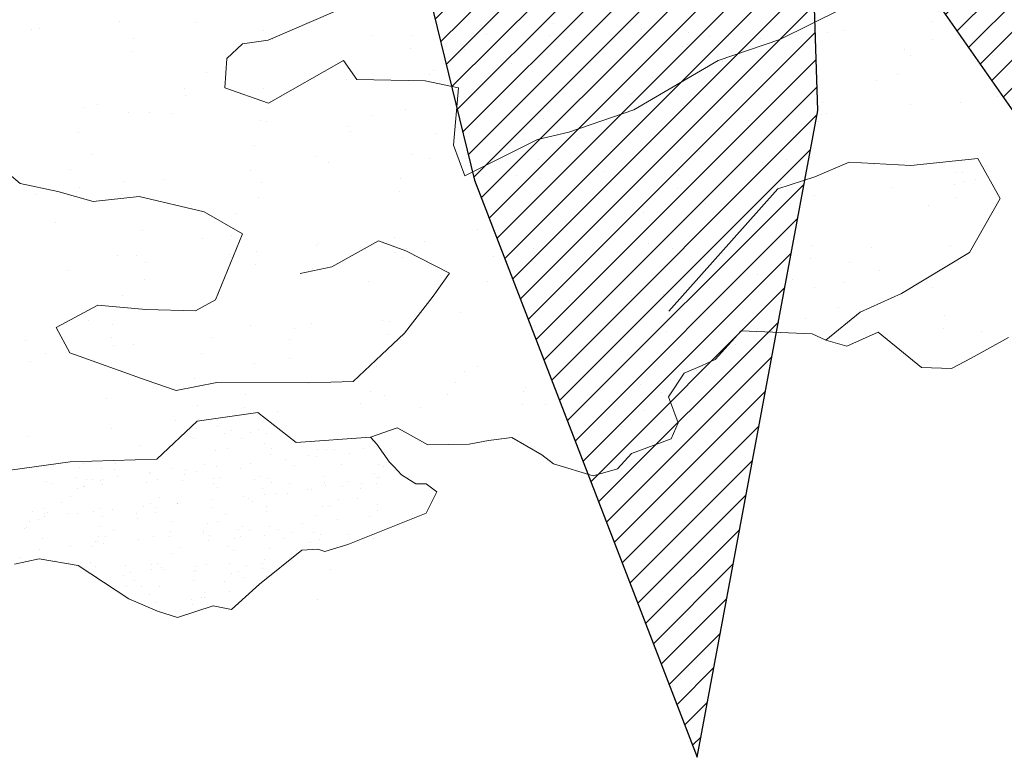
# Model space of a CAD drawing. Units: inches. Extents: x 1986 to 21484, y -1816 to 2016.
# Tile 52 of 85: x 3664.13 to 3671.752, y 1865.089 to 1870.798. Entities that reach past the tile are written whole.
import ezdxf

# ---------------------------------------------------------------- set-up
doc = ezdxf.new("R2010")
doc.units = ezdxf.units.IN
doc.layers.add('L-PLNT', color=84, linetype='Continuous', lineweight=13)
doc.layers.add('vfolhas', color=114, linetype='Continuous', lineweight=5)
for name, color, linetype in [('vfolha', 72, 'Continuous'), ('vfolha2', 110, 'Continuous'), ('vfolhas2', 102, 'Continuous')]:
    doc.layers.add(name, color=color, linetype=linetype)
pattern_1 = [(45, (-2446.5133113, 50.986076), (-0.004419417382, 0.004419417382), [])]

# ---------------------------------------------------------------- blocks, each defined once
blk = doc.blocks.new('arbusto_PB_verde_grande')
at = {"layer": 'vfolha2'}
h = blk.add_hatch(dxfattribs=at)
h.set_pattern_fill('ANSI31', color=256, scale=0.05, style=0)
h.set_pattern_definition(pattern_1)
h.paths.add_polyline_path([(-0.18963, 0.29704), (-0.08553, 0.20192), (-0.10785, 0.25007), (-0.13202, 0.31865), (-0.25096, 0.48479), (-0.44952, 0.5505), (-0.37946, 0.43789)])
h.paths.add_polyline_path([(0.07911, -0.4071), (0.08214, -0.50631), (0.17255, -0.6355), (0.18428, -0.44151), (0.14904, -0.29177), (0.02625, -0.03934), (0.03527, -0.25376)])
at = {"layer": 'vfolhas'}
h = blk.add_hatch(dxfattribs=at)
h.set_pattern_fill('ANSI31', color=256, scale=0.05, style=0)
h.set_pattern_definition(pattern_1)
h.paths.add_polyline_path([(-0.07279, 0.50669), (-0.18085, 0.65063), (-0.2334, 0.67253), (-0.20712, 0.53176), (-0.10785, 0.25007), (0.02625, -0.03934), (0.00028, 0.09048), (0.00816, 0.16241), (-0.04939, 0.29079)])
h.paths.add_polyline_path([(0.09902, 0.41929), (0.09372, 0.26573), (0.07906, 0.18814), (0.15506, 0.36901), (0.26606, 0.5505), (0.28356, 0.63504), (0.2485, 0.68819), (0.25145, 0.63504), (0.20178, 0.54426)])
h.paths.add_polyline_path([(0.12295, 0.24073), (0.047, 0.06233), (0.02625, -0.03934), (0.11122, 0.04358), (0.18428, 0.09364), (0.27478, 0.19376), (0.3215, 0.25323), (0.44129, 0.38467), (0.47634, 0.57866), (0.41789, 0.45347), (0.28939, 0.30954)])
h.paths.add_polyline_path([(0.58145, -0.03779), (0.70707, 0.01536), (0.78591, 0.04667), (0.74796, 0.06549), (0.62818, 0.08423), (0.52595, 0.09048), (0.39745, 0.04358), (0.02625, -0.03934), (0.25728, -0.03154), (0.43834, -0.0347)])
h.paths.add_polyline_path([(0.52022, -0.03647), (0.43834, -0.0347), (0.25728, -0.03154), (0.02625, -0.03934), (0.17964, -0.08515), (0.53768, -0.13167), (0.69541, -0.15357), (0.78591, -0.07852), (0.70413, -0.10042)])
h.paths.add_polyline_path([(0.27189, -0.21929), (0.14922, -0.14107), (0.02625, -0.03934), (0.15794, -0.31007), (0.29522, -0.42585), (0.41789, -0.49157), (0.56396, -0.56669), (0.5114, -0.48532), (0.39456, -0.34139)])
h.paths.add_polyline_path([(-0.05818, -0.47591), (-0.02312, -0.61984), (0.047, -0.80134), (0.08494, -0.59794), (0.07911, -0.4071), (0.03527, -0.25376), (0.02625, -0.03934), (-0.03773, -0.26001)])
h.paths.add_polyline_path([(-0.24218, 0.14054), (-0.11073, 0.06858), (0.02625, -0.03934), (-0.04235, 0.10871), (-0.21007, 0.23757), (-0.36485, 0.33145), (-0.47874, 0.40341), (-0.54303, 0.46288), (-0.49041, 0.33145), (-0.39408, 0.22192)])
at = {"layer": 'vfolha'}
for p, q in [((0.08494, -0.59794), (0.07911, -0.4071)), ((0.047, -0.80134), (0.08494, -0.59794)), ((-0.02312, -0.61984), (0.047, -0.80134))]:
    blk.add_line(p, q, dxfattribs=at)
at = {"layer": 'vfolha2'}
blk.add_line((0.08214, -0.50631), (0.17255, -0.6355), dxfattribs=at)
at = {"layer": 'vfolhas2'}
blk.add_line((-0.05818, -0.47591), (-0.02312, -0.61984), dxfattribs=at)
blk = doc.blocks.new('PLANT-SHRUB')
for p, q in [((2172.6241, 1903.2659), (2172.9437, 1903.1835)), ((2172.9437, 1903.1835), (2173.1087, 1903.1371)), ((2173.1087, 1903.1371), (2173.2736, 1902.9723)), ((2172.7447, 1903.0859), (2172.7447, 1903.0859)), ((2173.2736, 1902.9723), (2173.3303, 1902.5448)), ((2172.9389, 1902.8692), (2172.9389, 1902.8692)), ((2172.8652, 1902.8017), (2172.8652, 1902.8017)), ((2172.7867, 1902.5845), (2172.7867, 1902.5845)), ((2172.3937, 1902.5791), (2171.9348, 1902.4358)), ((2172.3937, 1902.5791), (2172.3937, 1902.5791)), ((2172.9961, 1902.4501), (2172.3937, 1902.5791)), ((2172.5128, 1902.5757), (2172.5128, 1902.5757)), ((2173.3303, 1902.5448), (2173.583, 1902.457)), ((2171.9348, 1902.4358), (2171.8488, 1902.0919)), ((2171.9348, 1902.4358), (2171.9348, 1902.4358)), ((2172.4674, 1902.4372), (2172.4674, 1902.4372)), ((2173.3259, 1902.3355), (2172.9961, 1902.4501)), ((2173.583, 1902.457), (2173.6695, 1902.312)), ((2173.583, 1902.457), (2173.583, 1902.457)), ((2173.6695, 1902.312), (2173.3259, 1902.3355)), ((2173.6695, 1902.312), (2173.7128, 1902.2026)), ((2172.9948, 1902.2058), (2172.9948, 1902.2058)), ((2171.8432, 1902.1697), (2171.8432, 1902.1697)), ((2171.9724, 1902.2009), (2171.9724, 1902.2009)), ((2172.0512, 1902.1424), (2172.0512, 1902.1424)), ((2172.1799, 1902.198), (2172.1799, 1902.198)), ((2173.4246, 1902.1957), (2173.4246, 1902.1957)), ((2173.7128, 1902.2026), (2174.0978, 1901.8122)), ((2171.8488, 1902.0919), (2172.2647, 1901.7766)), ((2171.8488, 1902.0919), (2171.8488, 1902.0919)), ((2172.0114, 1902.0906), (2172.0114, 1902.0906)), ((2172.046, 1902.051), (2172.046, 1902.051)), ((2172.1197, 1902.1185), (2172.1197, 1902.1185)), ((2172.3762, 1902.0996), (2172.3762, 1902.0996)), ((2173.256, 1902.0884), (2173.256, 1902.0884)), ((2173.6688, 1902.0864), (2173.6688, 1902.0864)), ((2172.919, 1902.0281), (2172.919, 1902.0281)), ((2173.1271, 1902.0007), (2173.1271, 1902.0007)), ((2174.8579, 1901.7985), (2174.9403, 1901.9952)), ((2174.9403, 1901.9952), (2175.0639, 1902.0501)), ((2175.0639, 1902.0501), (2175.3661, 1901.922)), ((2173.452, 1901.9579), (2173.452, 1901.9579)), ((2175.3661, 1901.922), (2175.5264, 1901.9357)), ((2175.5264, 1901.9357), (2175.7004, 1901.8442)), ((2171.4082, 1901.8444), (2171.4082, 1901.8444)), ((2173.9948, 1901.8865), (2173.9948, 1901.8865)), ((2174.0978, 1901.8122), (2174.3954, 1901.8351)), ((2174.2029, 1901.8591), (2174.2029, 1901.8591)), ((2174.3954, 1901.8351), (2174.5008, 1901.7985)), ((2175.7004, 1901.8442), (2175.8617, 1901.568)), ((2172.2647, 1901.7766), (2172.5945, 1901.4326)), ((2172.2647, 1901.7766), (2172.2647, 1901.7766)), ((2172.4877, 1901.8056), (2172.4877, 1901.8056)), ((2173.3211, 1901.7678), (2173.3211, 1901.7678)), ((2173.5338, 1901.7922), (2173.5338, 1901.7922)), ((2174.0978, 1901.8122), (2174.0978, 1901.8122)), ((2174.5008, 1901.7985), (2174.6427, 1901.7481)), ((2174.5278, 1901.8163), (2174.5278, 1901.8163)), ((2174.5562, 1901.7971), (2174.5562, 1901.7971)), ((2174.6427, 1901.7481), (2174.8579, 1901.7985)), ((2171.6482, 1901.6865), (2171.6482, 1901.6865)), ((2173.2475, 1901.7003), (2173.2475, 1901.7003)), ((2174.8703, 1901.7356), (2174.8703, 1901.7356)), ((2175.0707, 1901.7448), (2175.0707, 1901.7448)), ((2175.2787, 1901.7175), (2175.2787, 1901.7175)), ((2175.6036, 1901.6747), (2175.6036, 1901.6747)), ((2171.2193, 1901.586), (2171.2193, 1901.586)), ((2172.4639, 1901.5837), (2172.4639, 1901.5837)), ((2173.7085, 1901.5815), (2173.7085, 1901.5815)), ((2174.9532, 1901.5792), (2174.9532, 1901.5792)), ((2175.8617, 1901.568), (2175.88, 1901.4537)), ((2175.88, 1901.4537), (2175.9578, 1901.1974)), ((2171.3005, 1901.3679), (2171.3005, 1901.3679)), ((2171.9472, 1901.4308), (2171.9472, 1901.4308)), ((2172.5945, 1901.4326), (2172.867, 1901.3323)), ((2172.9696, 1901.4357), (2172.9696, 1901.4357)), ((2174.0491, 1901.3968), (2174.0491, 1901.3968)), ((2174.5226, 1901.417), (2174.5226, 1901.417)), ((2175.0953, 1901.3835), (2175.0953, 1901.3835)), ((2171.2268, 1901.3004), (2171.2268, 1901.3004)), ((2172.8497, 1901.3357), (2172.8497, 1901.3357)), ((2172.867, 1901.3323), (2173.1395, 1901.2034)), ((2173.1395, 1901.2034), (2174.4016, 1901.318)), ((2174.4016, 1901.318), (2174.4016, 1901.318)), ((2174.4489, 1901.3495), (2174.4489, 1901.3495)), ((2171.4747, 1901.1835), (2171.4747, 1901.1835)), ((2171.6827, 1901.1561), (2171.6827, 1901.1561)), ((2171.8572, 1901.1972), (2171.8572, 1901.1972)), ((2173.1018, 1901.1949), (2173.1018, 1901.1949)), ((2174.3464, 1901.1927), (2174.3464, 1901.1927)), ((2175.591, 1901.1904), (2175.591, 1901.1904)), ((2175.9578, 1901.1974), (2176.1044, 1901.0922)), ((2176.6676, 1901.1059), (2176.8415, 1901.17)), ((2176.8415, 1901.17), (2177.4505, 1900.9321)), ((2176.8415, 1901.17), (2176.8415, 1901.17)), ((2171.383, 1901.0744), (2171.383, 1901.0744)), ((2171.6886, 1901.0898), (2171.6886, 1901.0898)), ((2172.0077, 1901.1133), (2172.0077, 1901.1133)), ((2172.9332, 1901.0876), (2172.9332, 1901.0876)), ((2174.1779, 1901.0853), (2174.1779, 1901.0853)), ((2175.4225, 1901.083), (2175.4225, 1901.083)), ((2175.7241, 1901.0662), (2175.7241, 1901.0662)), ((2176.1044, 1901.0922), (2176.2326, 1901.0099)), ((2176.6859, 1901.0053), (2176.6676, 1901.1059)), ((2177.9118, 1901.0785), (2177.9118, 1901.0785)), ((2172.4625, 1901.0355), (2172.4625, 1901.0355)), ((2172.502, 1901.0171), (2172.502, 1901.0171)), ((2172.5505, 1901.0418), (2172.5505, 1901.0418)), ((2172.7586, 1901.0144), (2172.7586, 1901.0144)), ((2173.5087, 1901.0221), (2173.5087, 1901.0221)), ((2174.0511, 1900.985), (2174.0511, 1900.985)), ((2174.5311, 1901.027), (2174.5311, 1901.027)), ((2175.6105, 1900.9881), (2175.6105, 1900.9881)), ((2175.6504, 1900.9987), (2175.6504, 1900.9987)), ((2176.2326, 1901.0099), (2176.4707, 1900.7948)), ((2176.7454, 1900.9504), (2176.6859, 1901.0053)), ((2177.2732, 1901.034), (2177.2732, 1901.034)), ((2172.4283, 1900.9496), (2172.4283, 1900.9496)), ((2173.0835, 1900.9717), (2173.0835, 1900.9717)), ((2176.7774, 1900.8223), (2176.7454, 1900.9504)), ((2177.4505, 1900.9321), (2177.6154, 1900.8497)), ((2177.6791, 1900.9797), (2177.6791, 1900.9797)), ((2173.6264, 1900.9002), (2173.6264, 1900.9002)), ((2173.8344, 1900.8728), (2173.8344, 1900.8728)), ((2177.0704, 1900.8682), (2177.0704, 1900.8682)), ((2177.0998, 1900.8952), (2177.0998, 1900.8952)), ((2177.182, 1900.8875), (2177.182, 1900.8875)), ((2177.392, 1900.8776), (2177.392, 1900.8776)), ((2177.6154, 1900.8497), (2177.6428, 1900.7994)), ((2174.1593, 1900.83), (2174.1593, 1900.83)), ((2174.7022, 1900.7585), (2174.7022, 1900.7585)), ((2176.4707, 1900.7948), (2176.5302, 1900.6027)), ((2176.7774, 1900.7399), (2176.7774, 1900.8223)), ((2177.5804, 1900.7549), (2177.5804, 1900.7549)), ((2177.6428, 1900.7994), (2177.739, 1900.7216)), ((2174.9102, 1900.7312), (2174.9102, 1900.7312)), ((2175.2351, 1900.6884), (2175.2351, 1900.6884)), ((2176.7545, 1900.5203), (2176.7774, 1900.6896)), ((2176.7774, 1900.6896), (2176.7774, 1900.7399)), ((2176.8372, 1900.6844), (2176.8372, 1900.6844)), ((2176.9112, 1900.7224), (2176.9112, 1900.7224)), ((2176.9255, 1900.7154), (2176.9255, 1900.7154)), ((2176.9659, 1900.7376), (2176.9659, 1900.7376)), ((2177.0819, 1900.68), (2177.0819, 1900.68)), ((2177.1493, 1900.7229), (2177.1493, 1900.7229)), ((2177.3748, 1900.7395), (2177.3748, 1900.7395)), ((2177.5509, 1900.7279), (2177.5509, 1900.7279)), ((2177.5798, 1900.6791), (2177.5798, 1900.6791)), ((2177.6472, 1900.722), (2177.6472, 1900.722)), ((2177.739, 1900.7216), (2178.1577, 1900.6883)), ((2178.1577, 1900.6883), (2178.4507, 1900.6838)), ((2178.1577, 1900.6883), (2178.1577, 1900.6883)), ((2178.4507, 1900.6838), (2178.5331, 1900.5648)), ((2171.9221, 1900.6607), (2171.9221, 1900.6607)), ((2172.9445, 1900.6656), (2172.9445, 1900.6656)), ((2173.7034, 1900.6663), (2173.7034, 1900.6663)), ((2174.0239, 1900.6267), (2174.0239, 1900.6267)), ((2175.0701, 1900.6134), (2175.0701, 1900.6134)), ((2175.2526, 1900.6342), (2175.2526, 1900.6342)), ((2175.778, 1900.6169), (2175.778, 1900.6169)), ((2176.0925, 1900.6183), (2176.0925, 1900.6183)), ((2176.5302, 1900.6027), (2176.5531, 1900.534)), ((2176.8519, 1900.6479), (2176.8519, 1900.6479)), ((2176.9204, 1900.6735), (2176.9204, 1900.6735)), ((2177.0504, 1900.6564), (2177.0504, 1900.6564)), ((2177.2675, 1900.6278), (2177.2675, 1900.6278)), ((2177.3507, 1900.6168), (2177.3507, 1900.6168)), ((2178.061, 1900.6146), (2178.061, 1900.6146)), ((2178.0776, 1900.6782), (2178.0776, 1900.6782)), ((2172.0305, 1900.5851), (2172.0305, 1900.5851)), ((2172.1411, 1900.5829), (2172.1411, 1900.5829)), ((2173.3857, 1900.5806), (2173.3857, 1900.5806)), ((2173.6298, 1900.5988), (2173.6298, 1900.5988)), ((2174.6304, 1900.5784), (2174.6304, 1900.5784)), ((2175.875, 1900.5761), (2175.875, 1900.5761)), ((2175.986, 1900.5895), (2175.986, 1900.5895)), ((2176.311, 1900.5467), (2176.311, 1900.5467)), ((2176.5531, 1900.534), (2176.7545, 1900.4471)), ((2176.7722, 1900.5949), (2176.7722, 1900.5949)), ((2177.1196, 1900.5739), (2177.1196, 1900.5739)), ((2177.172, 1900.5794), (2177.172, 1900.5794)), ((2177.172, 1900.5794), (2177.172, 1900.5794)), ((2177.3918, 1900.5821), (2177.3918, 1900.5821)), ((2177.4807, 1900.5997), (2177.4807, 1900.5997)), ((2177.5904, 1900.5741), (2177.5904, 1900.5741)), ((2177.6978, 1900.5711), (2177.6978, 1900.5711)), ((2177.781, 1900.5602), (2177.781, 1900.5602)), ((2177.911, 1900.5431), (2177.911, 1900.5431)), ((2177.9994, 1900.576), (2177.9994, 1900.576)), ((2178.0315, 1900.5876), (2178.0315, 1900.5876)), ((2178.2181, 1900.5661), (2178.2181, 1900.5661)), ((2178.3643, 1900.5716), (2178.3643, 1900.5716)), ((2178.5331, 1900.5648), (2178.7987, 1900.4413)), ((2171.83, 1900.525), (2172.3365, 1900.371)), ((2176.7545, 1900.4471), (2176.7545, 1900.5203)), ((2176.7651, 1900.4781), (2176.7651, 1900.4781)), ((2176.8538, 1900.4753), (2176.8538, 1900.4753)), ((2177.2527, 1900.4546), (2177.2527, 1900.4546)), ((2177.2629, 1900.4772), (2177.2629, 1900.4772)), ((2177.7608, 1900.4763), (2177.7608, 1900.4763)), ((2178.1282, 1900.5145), (2178.1282, 1900.5145)), ((2178.2114, 1900.5035), (2178.2114, 1900.5035)), ((2178.2586, 1900.4754), (2178.2586, 1900.4754)), ((2178.3413, 1900.4864), (2178.3413, 1900.4864)), ((2178.5416, 1900.4743), (2178.5416, 1900.4743)), ((2178.5585, 1900.4578), (2178.5585, 1900.4578)), ((2176.7545, 1900.4471), (2177.201, 1900.0838)), ((2176.9558, 1900.4295), (2176.9558, 1900.4295)), ((2177.0619, 1900.4479), (2177.0619, 1900.4479)), ((2177.2233, 1900.4276), (2177.2233, 1900.4276)), ((2177.3647, 1900.4315), (2177.3647, 1900.4315)), ((2177.3868, 1900.4051), (2177.3868, 1900.4051)), ((2177.7965, 1900.4159), (2177.7965, 1900.4159)), ((2177.8724, 1900.4418), (2177.8724, 1900.4418)), ((2178.215, 1900.4106), (2178.215, 1900.4106)), ((2178.5121, 1900.4473), (2178.5121, 1900.4473)), ((2178.624, 1900.4126), (2178.624, 1900.4126)), ((2178.6417, 1900.4469), (2178.6417, 1900.4469)), ((2178.7987, 1900.4413), (2178.8765, 1900.2994)), ((2172.3365, 1900.371), (2172.7952, 1900.1643)), ((2174.9049, 1900.3156), (2174.9049, 1900.3156)), ((2177.0202, 1900.3226), (2177.0202, 1900.3226)), ((2177.5181, 1900.3217), (2177.5181, 1900.3217)), ((2177.7333, 1900.3143), (2177.7333, 1900.3143)), ((2177.9296, 1900.3336), (2177.9296, 1900.3336)), ((2178.0159, 1900.3208), (2178.0159, 1900.3208)), ((2178.127, 1900.3646), (2178.127, 1900.3646)), ((2178.1377, 1900.3063), (2178.1377, 1900.3063)), ((2178.353, 1900.3014), (2178.353, 1900.3014)), ((2178.5138, 1900.3199), (2178.5138, 1900.3199)), ((2178.8765, 1900.2994), (2178.9727, 1900.0798)), ((2172.4373, 1900.2654), (2172.4373, 1900.2654)), ((2173.232, 1900.2343), (2173.232, 1900.2343)), ((2173.4835, 1900.252), (2173.4835, 1900.252)), ((2174.5059, 1900.2569), (2174.5059, 1900.2569)), ((2174.8312, 1900.2481), (2174.8312, 1900.2481)), ((2176.4541, 1900.2834), (2176.4541, 1900.2834)), ((2177.0642, 1900.2818), (2177.0642, 1900.2818)), ((2177.1201, 1900.2333), (2177.1201, 1900.2333)), ((2177.1619, 1900.2714), (2177.1619, 1900.2714)), ((2177.2033, 1900.2223), (2177.2033, 1900.2223)), ((2177.4507, 1900.2788), (2177.4507, 1900.2788)), ((2177.5804, 1900.266), (2177.5804, 1900.266)), ((2177.7039, 1900.2873), (2177.7039, 1900.2873)), ((2177.9485, 1900.2779), (2177.9485, 1900.2779)), ((2177.9893, 1900.268), (2177.9893, 1900.268)), ((2178.0533, 1900.2971), (2178.0533, 1900.2971)), ((2178.4211, 1900.2524), (2178.4211, 1900.2524)), ((2178.4464, 1900.277), (2178.4464, 1900.277)), ((2178.4626, 1900.2635), (2178.4626, 1900.2635)), ((2178.8396, 1900.2471), (2178.8396, 1900.2471)), ((2172.779, 1900.1941), (2172.779, 1900.1941)), ((2172.7952, 1900.1643), (2173.5327, 1899.9936)), ((2174.0236, 1900.1919), (2174.0236, 1900.1919)), ((2175.2683, 1900.1896), (2175.2683, 1900.1896)), ((2175.5854, 1900.218), (2175.5854, 1900.218)), ((2176.5129, 1900.1873), (2176.5129, 1900.1873)), ((2176.6315, 1900.2047), (2176.6315, 1900.2047)), ((2177.3333, 1900.2052), (2177.3333, 1900.2052)), ((2177.5504, 1900.1766), (2177.5504, 1900.1766)), ((2177.6336, 1900.1657), (2177.6336, 1900.1657)), ((2177.6539, 1900.2096), (2177.6539, 1900.2096)), ((2177.7575, 1900.1851), (2177.7575, 1900.1851)), ((2177.7636, 1900.1485), (2177.7636, 1900.1485)), ((2178.1844, 1900.147), (2178.1844, 1900.147)), ((2178.2139, 1900.174), (2178.2139, 1900.174)), ((2178.7334, 1900.1707), (2178.7334, 1900.1707)), ((2178.8336, 1900.1611), (2178.8336, 1900.1611)), ((2172.6105, 1900.0867), (2172.6105, 1900.0867)), ((2173.8551, 1900.0845), (2173.8551, 1900.0845)), ((2175.0997, 1900.0822), (2175.0997, 1900.0822)), ((2176.3444, 1900.08), (2176.3444, 1900.08)), ((2177.201, 1900.0838), (2177.2584, 1899.7112)), ((2177.3547, 1900.1234), (2177.3547, 1900.1234)), ((2177.5447, 1900.1415), (2177.5447, 1900.1415)), ((2177.589, 1900.0777), (2177.589, 1900.0777)), ((2177.6317, 1900.076), (2177.6317, 1900.076)), ((2177.7865, 1900.1079), (2177.7865, 1900.1079)), ((2177.9808, 1900.12), (2177.9808, 1900.12)), ((2178.064, 1900.109), (2178.064, 1900.109)), ((2178.1295, 1900.0751), (2178.1295, 1900.0751)), ((2178.194, 1900.0919), (2178.194, 1900.0919)), ((2178.2049, 1900.1026), (2178.2049, 1900.1026)), ((2178.6139, 1900.1045), (2178.6139, 1900.1045)), ((2178.6274, 1900.0742), (2178.6274, 1900.0742)), ((2178.8336, 1900.0754), (2178.8336, 1900.0754)), ((2178.9727, 1900.0798), (2179.0826, 1899.6223)), ((2173.5327, 1899.9936), (2174.0183, 1899.7779)), ((2175.6521, 1899.9834), (2176.0107, 1900.0408)), ((2176.0107, 1900.0408), (2176.2545, 1900.0408)), ((2176.2545, 1900.0408), (2176.5556, 1900.0408)), ((2176.5556, 1900.0408), (2176.8138, 1899.8115)), ((2177.4057, 1900.0141), (2177.4057, 1900.0141)), ((2178.0253, 1900.0012), (2178.0253, 1900.0012)), ((2178.4111, 1900.0633), (2178.4111, 1900.0633)), ((2178.4943, 1900.0523), (2178.4943, 1900.0523)), ((2178.6243, 1900.0352), (2178.6243, 1900.0352)), ((2178.665, 1900.0067), (2178.665, 1900.0067)), ((2178.6945, 1900.0337), (2178.6945, 1900.0337)), ((2178.8414, 1900.0066), (2178.8414, 1900.0066)), ((2178.9246, 1899.9957), (2178.9246, 1899.9957)), ((2172.715, 1899.9854), (2172.715, 1899.9854)), ((2175.437, 1899.9405), (2175.6521, 1899.9834)), ((2175.5661, 1899.5822), (2175.437, 1899.9405)), ((2176.1063, 1899.9648), (2176.1063, 1899.9648)), ((2177.3762, 1899.9871), (2177.3762, 1899.9871)), ((2177.389, 1899.9214), (2177.389, 1899.9214)), ((2177.5703, 1899.958), (2177.5703, 1899.958)), ((2177.6555, 1899.9326), (2177.6555, 1899.9326)), ((2177.8868, 1899.9205), (2177.8868, 1899.9205)), ((2177.9792, 1899.96), (2177.9792, 1899.96)), ((2178.3847, 1899.9196), (2178.3847, 1899.9196)), ((2178.411, 1899.9444), (2178.411, 1899.9444)), ((2178.8295, 1899.9391), (2178.8295, 1899.9391)), ((2178.8825, 1899.9187), (2178.8825, 1899.9187)), ((2172.8106, 1899.8482), (2172.8106, 1899.8482)), ((2172.8842, 1899.9157), (2172.8842, 1899.9157)), ((2172.9193, 1899.8955), (2172.9193, 1899.8955)), ((2173.2579, 1899.9139), (2173.2579, 1899.9139)), ((2173.4659, 1899.8865), (2173.4659, 1899.8865)), ((2173.7908, 1899.8437), (2173.7908, 1899.8437)), ((2173.9987, 1899.8567), (2173.9987, 1899.8567)), ((2174.4334, 1899.8835), (2174.4334, 1899.8835)), ((2175.0449, 1899.8433), (2175.0449, 1899.8433)), ((2176.0327, 1899.8973), (2176.0327, 1899.8973)), ((2176.0673, 1899.8482), (2176.0673, 1899.8482)), ((2177.3215, 1899.8784), (2177.3215, 1899.8784)), ((2177.8194, 1899.8775), (2177.8194, 1899.8775)), ((2177.8568, 1899.8467), (2177.8568, 1899.8467)), ((2177.8862, 1899.8737), (2177.8862, 1899.8737)), ((2178.3172, 1899.8766), (2178.3172, 1899.8766)), ((2178.5059, 1899.8609), (2178.5059, 1899.8609)), ((2178.8151, 1899.8757), (2178.8151, 1899.8757)), ((2174.0183, 1899.7779), (2174.2342, 1899.6521)), ((2174.3337, 1899.7723), (2174.3337, 1899.7723)), ((2176.8138, 1899.8115), (2177.3301, 1899.3242)), ((2176.8138, 1899.8115), (2176.8138, 1899.8115)), ((2177.1468, 1899.8093), (2177.1468, 1899.8093)), ((2177.3446, 1899.8154), (2177.3446, 1899.8154)), ((2177.403, 1899.7821), (2177.403, 1899.7821)), ((2177.4863, 1899.7711), (2177.4863, 1899.7711)), ((2177.7764, 1899.7999), (2177.7764, 1899.7999)), ((2178.193, 1899.796), (2178.193, 1899.796)), ((2178.1949, 1899.7945), (2178.1949, 1899.7945)), ((2178.6038, 1899.7965), (2178.6038, 1899.7965)), ((2179.0356, 1899.7809), (2179.0356, 1899.7809)), ((2174.5417, 1899.7449), (2174.5417, 1899.7449)), ((2174.8666, 1899.7021), (2174.8666, 1899.7021)), ((2177.2584, 1899.7112), (2177.6456, 1899.4389)), ((2177.6162, 1899.754), (2177.6162, 1899.754)), ((2177.6976, 1899.7009), (2177.6976, 1899.7009)), ((2177.8334, 1899.7254), (2177.8334, 1899.7254)), ((2177.9166, 1899.7145), (2177.9166, 1899.7145)), ((2178.0466, 1899.6974), (2178.0466, 1899.6974)), ((2178.3374, 1899.7064), (2178.3374, 1899.7064)), ((2178.3668, 1899.7334), (2178.3668, 1899.7334)), ((2178.9865, 1899.7206), (2178.9865, 1899.7206)), ((2174.2342, 1899.6521), (2174.8367, 1899.4723)), ((2175.4095, 1899.6306), (2175.4095, 1899.6306)), ((2177.3078, 1899.614), (2177.3078, 1899.614)), ((2177.5025, 1899.6757), (2177.5025, 1899.6757)), ((2177.5602, 1899.65), (2177.5602, 1899.65)), ((2177.9692, 1899.6519), (2177.9692, 1899.6519)), ((2178.0004, 1899.6748), (2178.0004, 1899.6748)), ((2178.2637, 1899.6688), (2178.2637, 1899.6688)), ((2178.3469, 1899.6578), (2178.3469, 1899.6578)), ((2178.401, 1899.6364), (2178.401, 1899.6364)), ((2178.4769, 1899.6407), (2178.4769, 1899.6407)), ((2178.4982, 1899.6739), (2178.4982, 1899.6739)), ((2178.694, 1899.6121), (2178.694, 1899.6121)), ((2178.8194, 1899.631), (2178.8194, 1899.631)), ((2178.9961, 1899.673), (2178.9961, 1899.673)), ((2179.0826, 1899.6223), (2179.2664, 1899.3776)), ((2173.063, 1899.5798), (2173.063, 1899.5798)), ((2174.0857, 1899.5649), (2174.0857, 1899.5649)), ((2174.3076, 1899.5776), (2174.3076, 1899.5776)), ((2175.5522, 1899.5753), (2175.5522, 1899.5753)), ((2175.6664, 1899.3816), (2175.5661, 1899.5822)), ((2175.6175, 1899.6032), (2175.6175, 1899.6032)), ((2175.9425, 1899.5605), (2175.9425, 1899.5605)), ((2176.7969, 1899.573), (2176.7969, 1899.573)), ((2177.2341, 1899.5465), (2177.2341, 1899.5465)), ((2177.5291, 1899.5465), (2177.5291, 1899.5465)), ((2177.5586, 1899.5735), (2177.5586, 1899.5735)), ((2178.0415, 1899.5708), (2178.0415, 1899.5708)), ((2178.1782, 1899.5606), (2178.1782, 1899.5606)), ((2178.7772, 1899.6012), (2178.7772, 1899.6012)), ((2178.8179, 1899.5661), (2178.8179, 1899.5661)), ((2178.8474, 1899.5931), (2178.8474, 1899.5931)), ((2178.857, 1899.5818), (2178.857, 1899.5818)), ((2178.9072, 1899.5841), (2178.9072, 1899.5841)), ((2179.1244, 1899.5555), (2179.1244, 1899.5555)), ((2173.4583, 1899.4819), (2173.4583, 1899.4819)), ((2174.012, 1899.4974), (2174.012, 1899.4974)), ((2174.4807, 1899.4868), (2174.4807, 1899.4868)), ((2174.8367, 1899.4723), (2174.7378, 1899.2387)), ((2175.6349, 1899.5328), (2175.6349, 1899.5328)), ((2176.4853, 1899.489), (2176.4853, 1899.489)), ((2176.6934, 1899.4616), (2176.6934, 1899.4616)), ((2177.6903, 1899.4772), (2177.6903, 1899.4772)), ((2177.7577, 1899.5202), (2177.7577, 1899.5202)), ((2177.7663, 1899.4918), (2177.7663, 1899.4918)), ((2178.1848, 1899.4865), (2178.1848, 1899.4865)), ((2178.1881, 1899.4763), (2178.1881, 1899.4763)), ((2178.2555, 1899.5192), (2178.2555, 1899.5192)), ((2178.5937, 1899.4884), (2178.5937, 1899.4884)), ((2178.686, 1899.4754), (2178.686, 1899.4754)), ((2178.7534, 1899.5183), (2178.7534, 1899.5183)), ((2179.0255, 1899.4729), (2179.0255, 1899.4729)), ((2179.1838, 1899.4745), (2179.1838, 1899.4745)), ((2175.5602, 1899.4479), (2175.5602, 1899.4479)), ((2176.6063, 1899.4346), (2176.6063, 1899.4346)), ((2177.0183, 1899.4188), (2177.0183, 1899.4188)), ((2177.6287, 1899.4395), (2177.6287, 1899.4395)), ((2177.6456, 1899.4389), (2178.0759, 1899.4389)), ((2178.0759, 1899.4389), (2178.5778, 1898.9946)), ((2178.0759, 1899.4389), (2178.0759, 1899.4389)), ((2178.6588, 1899.4203), (2178.6588, 1899.4203)), ((2178.7082, 1899.4006), (2178.7082, 1899.4006)), ((2176.068, 1899.2812), (2175.6664, 1899.3816)), ((2177.3301, 1899.3242), (2177.6026, 1899.1523)), ((2177.5612, 1899.3473), (2177.5612, 1899.3473)), ((2177.7692, 1899.32), (2177.7692, 1899.32)), ((2178.3909, 1899.3283), (2178.3909, 1899.3283)), ((2178.8094, 1899.323), (2178.8094, 1899.323)), ((2179.2183, 1899.325), (2179.2183, 1899.325)), ((2179.2664, 1899.3776), (2179.4358, 1899.2769)), ((2174.7378, 1899.2387), (2174.4051, 1898.9421)), ((2176.2831, 1899.1523), (2176.068, 1899.2812)), ((2178.0941, 1899.2772), (2178.0941, 1899.2772)), ((2178.3295, 1899.2462), (2178.3295, 1899.2462)), ((2178.3691, 1899.2735), (2178.3691, 1899.2735)), ((2178.4903, 1899.2659), (2178.4903, 1899.2659)), ((2178.5093, 1899.2632), (2178.5093, 1899.2632)), ((2178.5197, 1899.2929), (2178.5197, 1899.2929)), ((2178.867, 1899.2726), (2178.867, 1899.2726)), ((2179.1394, 1899.28), (2179.1394, 1899.28)), ((2179.3648, 1899.2717), (2179.3648, 1899.2717)), ((2173.7008, 1899.191), (2173.7008, 1899.191)), ((2174.9455, 1899.1888), (2174.9455, 1899.1888)), ((2175.2872, 1899.2141), (2175.2872, 1899.2141)), ((2176.1901, 1899.1865), (2176.1901, 1899.1865)), ((2176.8363, 1899.182), (2176.8363, 1899.182)), ((2177.4347, 1899.1842), (2177.4347, 1899.1842)), ((2178.4356, 1899.1957), (2178.4356, 1899.1957)), ((2178.5466, 1899.2176), (2178.5466, 1899.2176)), ((2178.5837, 1899.1804), (2178.5837, 1899.1804)), ((2178.6298, 1899.2067), (2178.6298, 1899.2067)), ((2178.637, 1899.2057), (2178.637, 1899.2057)), ((2178.6794, 1899.182), (2178.6794, 1899.182)), ((2178.7598, 1899.1895), (2178.7598, 1899.1895)), ((2178.845, 1899.1783), (2178.845, 1899.1783)), ((2178.977, 1899.161), (2178.977, 1899.161)), ((2179.0155, 1899.1648), (2179.0155, 1899.1648)), ((2173.5323, 1899.0837), (2173.5323, 1899.0837)), ((2173.6142, 1899.1329), (2173.6142, 1899.1329)), ((2173.9736, 1899.0866), (2173.9736, 1899.0866)), ((2174.7769, 1899.0814), (2174.7769, 1899.0814)), ((2175.2135, 1899.1466), (2175.2135, 1899.1466)), ((2176.0216, 1899.0791), (2176.0216, 1899.0791)), ((2176.0421, 1899.0781), (2176.0421, 1899.0781)), ((2177.6026, 1899.1523), (2177.7173, 1898.9373)), ((2178.6243, 1899.118), (2178.6243, 1899.118)), ((2178.9709, 1899.1256), (2178.9709, 1899.1256)), ((2179.0003, 1899.1526), (2179.0003, 1899.1526)), ((2179.0602, 1899.15), (2179.0602, 1899.15)), ((2179.1221, 1899.1171), (2179.1221, 1899.1171)), ((2179.1699, 1899.1355), (2179.1699, 1899.1355)), ((2179.1901, 1899.1329), (2179.1901, 1899.1329)), ((2175.0197, 1899.0732), (2175.0197, 1899.0732)), ((2177.1216, 1899.0392), (2177.1216, 1899.0392)), ((2177.2662, 1899.0769), (2177.2662, 1899.0769)), ((2178.1678, 1899.0259), (2178.1678, 1899.0259)), ((2178.5108, 1899.0746), (2178.5108, 1899.0746)), ((2178.5569, 1899.0751), (2178.5569, 1899.0751)), ((2178.7993, 1899.015), (2178.7993, 1899.015)), ((2179.0547, 1899.0742), (2179.0547, 1899.0742)), ((2174.4051, 1898.9421), (2174.5579, 1898.7264)), ((2177.7173, 1898.9373), (2178.0041, 1898.3784)), ((2177.7173, 1898.9373), (2177.7173, 1898.9373)), ((2178.5778, 1898.9946), (2179.0654, 1898.6507)), ((2178.8117, 1898.9797), (2178.8117, 1898.9797)), ((2176.8998, 1898.8513), (2176.3979, 1898.622)), ((2176.4886, 1898.8634), (2176.4886, 1898.8634)), ((2176.8998, 1898.8513), (2176.8998, 1898.8513)), ((2177.0719, 1898.8083), (2176.8998, 1898.8513)), ((2173.9652, 1898.786), (2173.9652, 1898.786)), ((2174.8157, 1898.7821), (2174.8157, 1898.7821)), ((2176.415, 1898.7959), (2176.415, 1898.7959)), ((2177.3444, 1898.5361), (2177.0719, 1898.8083)), ((2178.0378, 1898.8312), (2178.0378, 1898.8312)), ((2174.1732, 1898.7586), (2174.1732, 1898.7586)), ((2174.4555, 1898.7167), (2174.4555, 1898.7167)), ((2174.4981, 1898.7158), (2174.4981, 1898.7158)), ((2174.5579, 1898.7264), (2174.9357, 1898.358)), ((2175.041, 1898.6443), (2175.041, 1898.6443)), ((2175.535, 1898.6778), (2175.535, 1898.6778)), ((2176.3979, 1898.622), (2176.4983, 1898.2924)), ((2176.3979, 1898.622), (2176.3979, 1898.622)), ((2176.5812, 1898.6645), (2176.5812, 1898.6645)), ((2177.6036, 1898.6694), (2177.6036, 1898.6694)), ((2178.683, 1898.6305), (2178.683, 1898.6305)), ((2175.2294, 1898.5745), (2175.2294, 1898.5745)), ((2175.249, 1898.6169), (2175.249, 1898.6169)), ((2175.574, 1898.5742), (2175.574, 1898.5742)), ((2176.4741, 1898.5722), (2176.4741, 1898.5722)), ((2177.7187, 1898.57), (2177.7187, 1898.57)), ((2176.1168, 1898.5027), (2176.1168, 1898.5027)), ((2176.3249, 1898.4753), (2176.3249, 1898.4753)), ((2177.5942, 1898.2576), (2177.3444, 1898.5361)), ((2177.6901, 1898.5126), (2177.6901, 1898.5126)), ((2174.3943, 1898.396), (2174.3943, 1898.396)), ((2174.468, 1898.4635), (2174.468, 1898.4635)), ((2176.0172, 1898.4313), (2176.0172, 1898.4313)), ((2176.6498, 1898.4325), (2176.6498, 1898.4325)), ((2177.6164, 1898.4451), (2177.6164, 1898.4451)), ((2174.9357, 1898.358), (2174.9087, 1898.1783)), ((2177.1927, 1898.3611), (2177.1927, 1898.3611)), ((2177.4007, 1898.3337), (2177.4007, 1898.3337)), ((2178.0041, 1898.3784), (2177.9468, 1898.1635)), ((2174.9946, 1898.3031), (2174.9946, 1898.3031)), ((2176.017, 1898.308), (2176.017, 1898.308)), ((2176.4983, 1898.2924), (2176.7851, 1897.8625)), ((2177.0964, 1898.2691), (2177.0964, 1898.2691)), ((2177.9468, 1898.1635), (2177.5942, 1898.2576)), ((2177.7256, 1898.2909), (2177.7256, 1898.2909)), ((2178.1426, 1898.2558), (2178.1426, 1898.2558)), ((2174.6227, 1898.188), (2174.6227, 1898.188)), ((2174.9087, 1898.1783), (2175.5585, 1898.022)), ((2175.8673, 1898.1857), (2175.8673, 1898.1857)), ((2177.112, 1898.1834), (2177.112, 1898.1834)), ((2178.2685, 1898.2194), (2178.2685, 1898.2194)), ((2175.6695, 1898.1127), (2175.6695, 1898.1127)), ((2175.5585, 1898.022), (2175.7246, 1897.7028)), ((2175.5958, 1898.0452), (2175.5958, 1898.0452)), ((2175.6988, 1898.0783), (2175.6988, 1898.0783)), ((2176.9434, 1898.0761), (2176.9434, 1898.0761)), ((2177.2186, 1898.0806), (2177.2186, 1898.0806)), ((2178.1881, 1898.0738), (2178.1881, 1898.0738)), ((2175.2263, 1897.6645), (2174.5236, 1897.9199)), ((2175.5098, 1897.9077), (2175.5098, 1897.9077)), ((2176.556, 1897.8944), (2176.556, 1897.8944)), ((2176.7851, 1897.8625), (2177.0719, 1897.6476)), ((2177.5784, 1897.8993), (2177.5784, 1897.8993)), ((2176.8709, 1897.7619), (2176.8709, 1897.7619)), ((2175.198, 1897.6807), (2175.198, 1897.6807)), ((2175.3924, 1897.5496), (2175.2263, 1897.6645)), ((2175.7246, 1897.7028), (2175.5585, 1897.5496)), ((2176.7972, 1897.6944), (2176.7972, 1897.6944)), ((2177.0719, 1897.6476), (2177.2154, 1897.4039)), ((2175.2055, 1897.5879), (2175.2055, 1897.5879)), ((2176.1513, 1897.5714), (2176.1513, 1897.5714)), ((2177.3959, 1897.5692), (2177.3959, 1897.5692)), ((2175.5585, 1897.5496), (2175.3924, 1897.5496)), ((2175.7483, 1897.5164), (2175.7483, 1897.5164)), ((2175.9564, 1897.489), (2175.9564, 1897.489)), ((2175.9918, 1897.5379), (2175.9918, 1897.5379)), ((2177.0713, 1897.499), (2177.0713, 1897.499)), ((2176.2813, 1897.4462), (2176.2813, 1897.4462)), ((2177.2154, 1897.4039), (2177.3875, 1897.1603)), ((2176.3994, 1897.3299), (2176.3994, 1897.3299)), ((2176.8242, 1897.3748), (2176.8242, 1897.3748)), ((2177.0322, 1897.3474), (2177.0322, 1897.3474)), ((2177.3571, 1897.3046), (2177.3571, 1897.3046)), ((2175.5445, 1897.1849), (2175.5445, 1897.1849)), ((2176.7892, 1897.1826), (2176.7892, 1897.1826)), ((2176.5308, 1897.1243), (2176.5308, 1897.1243)), ((2177.3875, 1897.1603), (2177.4161, 1896.9167)), ((2176.6206, 1897.0752), (2176.6206, 1897.0752)), ((2175.9781, 1896.9438), (2175.9781, 1896.9438)), ((2176.0517, 1897.0113), (2176.0517, 1897.0113)), ((2175.9666, 1896.7678), (2175.9666, 1896.7678)), ((2176.4557, 1896.3885), (2176.4557, 1896.3885)), ((2176.5056, 1896.3542), (2176.5056, 1896.3542))]:
    blk.add_line(p, q)

msp = doc.modelspace()

# ---------------------------------------------------------------- block references
at = {"layer": 'L-PLNT', "rotation": 223.1883365522388}
msp.add_blockref('PLANT-SHRUB', (3953.27, 4742.9646), dxfattribs=at)
at = {"layer": 'L-PLNT', "xscale": 24.60366729364114, "yscale": 24.60366729364114, "zscale": 24.60366729364114}
msp.add_blockref('arbusto_PB_verde_grande', (3668.2184, 1884.8051), dxfattribs=at)

doc.saveas('drawing.dxf')
